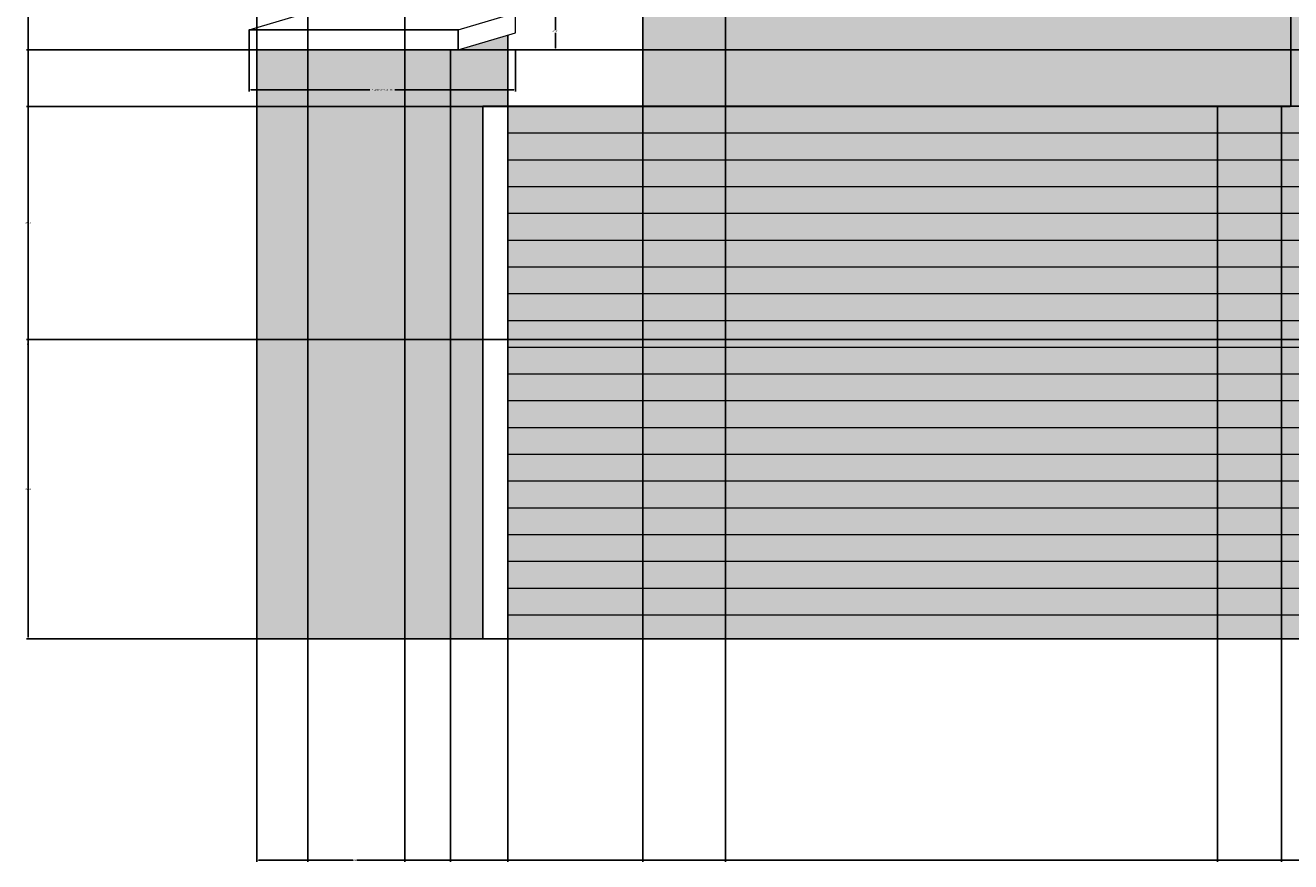
# Model space of a CAD drawing. Units: feet. Extents: x 2926 to 4178, y 965 to 1469.
# Tile 1 of 9: x 2926 to 3068, y 965 to 1059. Entities that reach past the tile are written whole.
import ezdxf

# ---------------------------------------------------------------- set-up
doc = ezdxf.new("R2010")
doc.units = ezdxf.units.FT
for name, color, linetype, lineweight in [('A-ANNO-DIMS', 2, 'Continuous', 18), ('A-ELEV', 7, 'Continuous', 25), ('A-ELEV-DETL', 8, 'Continuous', 18), ('A-ELEV-PATT', 9, 'Continuous', 13)]:
    doc.layers.add(name, color=color, linetype=linetype, lineweight=lineweight)
doc.styles.get("Standard").update_dxf_attribs({"font": 'arial.ttf'})
doc.dimstyles.get("Standard").update_dxf_attribs({"dimtxt": 0.18, "dimasz": 0.18, "dimexe": 0.18, "dimexo": 0.0625, "dimgap": 0.09, "dimtad": 0, "dimtih": 1, "dimtoh": 1, "dimdec": 1, "dimzin": 0, "dimdsep": 46, "dimlunit": 3, "dimtxsty": 'Standard', "dimcen": 0.09, "dimadec": 0, "dimazin": 0, "dimtfac": 1, "dimtdec": 1, "dimtofl": 0, "dimtmove": 0, "dimatfit": 3, "dimfxl": 1, "dimtolj": 1, "dimtzin": 0, "dimarcsym": 0})

# ---------------------------------------------------------------- blocks, each defined once
blk = doc.blocks.new('PILLAR-CAP-A')
for p, q in [((0, 2.25), (6.42, 4.14)), ((0, 2.25), (6.42, 4.14)), ((29.85, 4.14), (6.42, 4.14)), ((29.85, 4.14), (6.42, 4.14)), ((23.43, 2.25), (29.85, 4.14)), ((23.43, 2.25), (29.85, 4.14)), ((29.85, 1.89), (29.85, 4.14)), ((29.85, 1.89), (29.85, 4.14)), ((23.43, 0), (29.85, 1.89)), ((23.43, 0), (29.85, 1.89))]:
    blk.add_line(p, q)
blk = doc.blocks.new('*D6')
at = {"layer": 'A-ANNO-DIMS', "color": 0, "lineweight": -2, "transparency": 16777216}
for p, q in [((2951.55, 1056.26), (2951.55, 1051.66)), ((2981.4, 1056.26), (2981.4, 1051.66)), ((2951.73, 1051.84), (2965.07, 1051.84)), ((2981.22, 1051.84), (2967.88, 1051.84))]:
    blk.add_line(p, q, dxfattribs=at)
at = {"layer": 'A-ANNO-DIMS', "color": 0, "transparency": 16777216}
for points in [[(2951.73, 1051.87), (2951.73, 1051.81), (2951.55, 1051.84)], [(2981.22, 1051.87), (2981.22, 1051.81), (2981.4, 1051.84)]]:
    blk.add_solid(points, dxfattribs=at)
at = {"layer": 'Defpoints', "color": 0, "transparency": 16777216}
for p in [(2951.55, 1056.32), (2981.4, 1056.32), (2981.4, 1051.84)]:
    blk.add_point(p, dxfattribs=at)
at = {"layer": 'A-ANNO-DIMS', "color": 0, "transparency": 16777216, "insert": (2966.48, 1051.84), "char_height": 0.18, "attachment_point": 5}
blk.add_mtext('\\A1;PILLAR CAP A 30 TYP.', dxfattribs=at)
blk = doc.blocks.new('*D7')
at = {"layer": 'A-ANNO-DIMS', "color": 0, "lineweight": -2, "transparency": 16777216}
for p, q in [((2981.46, 1060.46), (2986.06, 1060.46)), ((2985.88, 1060.28), (2985.88, 1058.57)), ((2985.88, 1056.5), (2985.88, 1058.21)), ((2981.46, 1056.32), (2986.06, 1056.32))]:
    blk.add_line(p, q, dxfattribs=at)
at = {"layer": 'A-ANNO-DIMS', "color": 0, "transparency": 16777216}
for points in [[(2985.85, 1060.28), (2985.91, 1060.28), (2985.88, 1060.46)], [(2985.85, 1056.5), (2985.91, 1056.5), (2985.88, 1056.32)]]:
    blk.add_solid(points, dxfattribs=at)
at = {"layer": 'Defpoints', "color": 0, "transparency": 16777216}
for p in [(2981.4, 1060.46), (2985.88, 1060.46), (2981.4, 1056.32)]:
    blk.add_point(p, dxfattribs=at)
at = {"layer": 'A-ANNO-DIMS', "color": 0, "transparency": 16777216, "insert": (2985.88, 1058.39), "char_height": 0.18, "attachment_point": 5}
blk.add_mtext('\\A1;4 TYP.', dxfattribs=at)
blk = doc.blocks.new('*D12')
at = {"layer": 'A-ANNO-DIMS', "color": 0, "lineweight": -2, "transparency": 16777216}
for p, q in [((3335.85, 1023.86), (2926.57, 1023.86)), ((2926.75, 1023.68), (2926.75, 1007.27)), ((2926.75, 990.5), (2926.75, 1006.91)), ((2952.34, 990.32), (2926.57, 990.32))]:
    blk.add_line(p, q, dxfattribs=at)
at = {"layer": 'A-ANNO-DIMS', "color": 0, "transparency": 16777216}
for points in [[(2926.72, 1023.68), (2926.78, 1023.68), (2926.75, 1023.86)], [(2926.72, 990.5), (2926.78, 990.5), (2926.75, 990.32)]]:
    blk.add_solid(points, dxfattribs=at)
at = {"layer": 'Defpoints', "color": 0, "transparency": 16777216}
for p in [(2926.75, 1023.86), (3335.91, 1023.86), (2952.4, 990.32)]:
    blk.add_point(p, dxfattribs=at)
at = {"layer": 'A-ANNO-DIMS', "color": 0, "transparency": 16777216, "insert": (2926.75, 1007.09), "char_height": 0.18, "attachment_point": 5}
blk.add_mtext('\\A1;33.53', dxfattribs=at)
blk = doc.blocks.new('*D13')
at = {"layer": 'A-ANNO-DIMS', "color": 0, "lineweight": -2, "transparency": 16777216}
for p, q in [((3068.25, 1049.98), (2926.57, 1049.98)), ((2926.75, 1049.8), (2926.75, 1037.1)), ((2926.75, 1024.04), (2926.75, 1036.74)), ((3335.85, 1023.86), (2926.57, 1023.86))]:
    blk.add_line(p, q, dxfattribs=at)
at = {"layer": 'A-ANNO-DIMS', "color": 0, "transparency": 16777216}
for points in [[(2926.72, 1049.8), (2926.78, 1049.8), (2926.75, 1049.98)], [(2926.72, 1024.04), (2926.78, 1024.04), (2926.75, 1023.86)]]:
    blk.add_solid(points, dxfattribs=at)
at = {"layer": 'Defpoints', "color": 0, "transparency": 16777216}
for p in [(2926.75, 1049.98), (3068.31, 1049.98), (3335.91, 1023.86)]:
    blk.add_point(p, dxfattribs=at)
at = {"layer": 'A-ANNO-DIMS', "color": 0, "transparency": 16777216, "insert": (2926.75, 1036.92), "char_height": 0.18, "attachment_point": 5}
blk.add_mtext('\\A1;26.13', dxfattribs=at)
blk = doc.blocks.new('*D14')
at = {"layer": 'A-ANNO-DIMS', "color": 0, "lineweight": -2, "transparency": 16777216}
for p, q in [((3068.25, 1092.04), (2926.57, 1092.04)), ((2926.75, 1091.86), (2926.75, 1071.2)), ((2926.75, 1050.16), (2926.75, 1070.83)), ((3068.25, 1049.98), (2926.57, 1049.98))]:
    blk.add_line(p, q, dxfattribs=at)
at = {"layer": 'A-ANNO-DIMS', "color": 0, "transparency": 16777216}
for points in [[(2926.72, 1091.86), (2926.78, 1091.86), (2926.75, 1092.04)], [(2926.72, 1050.16), (2926.78, 1050.16), (2926.75, 1049.98)]]:
    blk.add_solid(points, dxfattribs=at)
at = {"layer": 'Defpoints', "color": 0, "transparency": 16777216}
for p in [(2926.75, 1092.04), (3068.31, 1092.04), (3068.31, 1049.98)]:
    blk.add_point(p, dxfattribs=at)
at = {"layer": 'A-ANNO-DIMS', "color": 0, "transparency": 16777216, "insert": (2926.75, 1071.01), "char_height": 0.18, "attachment_point": 5}
blk.add_mtext('\\A1;42.06', dxfattribs=at)
blk = doc.blocks.new('*D22')
at = {"layer": 'A-ANNO-DIMS', "color": 0, "lineweight": -2, "transparency": 16777216}
for p, q in [((2952.4, 1056.38), (2952.4, 1468.62)), ((2952.58, 1468.44), (3009.97, 1468.44)), ((3068.13, 1468.44), (3010.74, 1468.44)), ((3068.31, 1050.05), (3068.31, 1468.62))]:
    blk.add_line(p, q, dxfattribs=at)
at = {"layer": 'A-ANNO-DIMS', "color": 0, "transparency": 16777216}
for points in [[(2952.58, 1468.47), (2952.58, 1468.41), (2952.4, 1468.44)], [(3068.13, 1468.47), (3068.13, 1468.41), (3068.31, 1468.44)]]:
    blk.add_solid(points, dxfattribs=at)
at = {"layer": 'Defpoints', "color": 0, "transparency": 16777216}
for p in [(3068.31, 1468.44), (2952.4, 1056.32), (3068.31, 1049.98)]:
    blk.add_point(p, dxfattribs=at)
at = {"layer": 'A-ANNO-DIMS', "color": 0, "transparency": 16777216, "insert": (3010.36, 1468.44), "char_height": 0.18, "attachment_point": 5}
blk.add_mtext('\\A1;115.9', dxfattribs=at)
blk = doc.blocks.new('*D23')
at = {"layer": 'A-ANNO-DIMS', "color": 0, "lineweight": -2, "transparency": 16777216}
for p, q in [((3068.31, 1050.05), (3068.31, 1468.62)), ((3068.49, 1468.44), (3099.11, 1468.44)), ((3130.51, 1468.44), (3099.9, 1468.44)), ((3130.69, 1050.05), (3130.69, 1468.62))]:
    blk.add_line(p, q, dxfattribs=at)
at = {"layer": 'A-ANNO-DIMS', "color": 0, "transparency": 16777216}
for points in [[(3068.49, 1468.47), (3068.49, 1468.41), (3068.31, 1468.44)], [(3130.51, 1468.47), (3130.51, 1468.41), (3130.69, 1468.44)]]:
    blk.add_solid(points, dxfattribs=at)
at = {"layer": 'Defpoints', "color": 0, "transparency": 16777216}
for p in [(3130.69, 1468.44), (3068.31, 1049.98), (3130.69, 1049.98)]:
    blk.add_point(p, dxfattribs=at)
at = {"layer": 'A-ANNO-DIMS', "color": 0, "transparency": 16777216, "insert": (3099.5, 1468.44), "char_height": 0.18, "attachment_point": 5}
blk.add_mtext('\\A1;62.38', dxfattribs=at)
blk = doc.blocks.new('*D50')
at = {"layer": 'A-ANNO-DIMS', "color": 0, "lineweight": -2, "transparency": 16777216}
for p, q in [((2952.4, 1171.83), (2952.4, 965.34)), ((2958.11, 1170.16), (2958.11, 965.34)), ((2952.58, 965.52), (2954.87, 965.52)), ((2957.93, 965.52), (2955.65, 965.52))]:
    blk.add_line(p, q, dxfattribs=at)
at = {"layer": 'A-ANNO-DIMS', "color": 0, "transparency": 16777216}
for points in [[(2952.58, 965.55), (2952.58, 965.49), (2952.4, 965.52)], [(2957.93, 965.55), (2957.93, 965.49), (2958.11, 965.52)]]:
    blk.add_solid(points, dxfattribs=at)
at = {"layer": 'Defpoints', "color": 0, "transparency": 16777216}
for p in [(2952.4, 1171.9), (2958.11, 1170.22), (2958.11, 965.52)]:
    blk.add_point(p, dxfattribs=at)
at = {"layer": 'A-ANNO-DIMS', "color": 0, "transparency": 16777216, "insert": (2955.26, 965.52), "char_height": 0.18, "attachment_point": 5}
blk.add_mtext('\\A1;5.712', dxfattribs=at)
blk = doc.blocks.new('*D51')
at = {"layer": 'A-ANNO-DIMS', "color": 0, "lineweight": -2, "transparency": 16777216}
for p, q in [((2958.11, 1170.16), (2958.11, 965.34)), ((2968.99, 1170.16), (2968.99, 965.34)), ((2958.29, 965.52), (2963.11, 965.52)), ((2968.81, 965.52), (2963.99, 965.52))]:
    blk.add_line(p, q, dxfattribs=at)
at = {"layer": 'A-ANNO-DIMS', "color": 0, "transparency": 16777216}
for points in [[(2958.29, 965.55), (2958.29, 965.49), (2958.11, 965.52)], [(2968.81, 965.55), (2968.81, 965.49), (2968.99, 965.52)]]:
    blk.add_solid(points, dxfattribs=at)
at = {"layer": 'Defpoints', "color": 0, "transparency": 16777216}
for p in [(2958.11, 1170.22), (2968.99, 1170.22), (2968.99, 965.52)]:
    blk.add_point(p, dxfattribs=at)
at = {"layer": 'A-ANNO-DIMS', "color": 0, "transparency": 16777216, "insert": (2963.55, 965.52), "char_height": 0.18, "attachment_point": 5}
blk.add_mtext('\\A1;10.871', dxfattribs=at)
blk = doc.blocks.new('*D52')
at = {"layer": 'A-ANNO-DIMS', "color": 0, "lineweight": -2, "transparency": 16777216}
for p, q in [((2968.99, 1170.16), (2968.99, 965.34)), ((2995.67, 1170.16), (2995.67, 965.34)), ((2969.17, 965.52), (2981.86, 965.52)), ((2995.49, 965.52), (2982.79, 965.52))]:
    blk.add_line(p, q, dxfattribs=at)
at = {"layer": 'A-ANNO-DIMS', "color": 0, "transparency": 16777216}
for points in [[(2969.17, 965.55), (2969.17, 965.49), (2968.99, 965.52)], [(2995.49, 965.55), (2995.49, 965.49), (2995.67, 965.52)]]:
    blk.add_solid(points, dxfattribs=at)
at = {"layer": 'Defpoints', "color": 0, "transparency": 16777216}
for p in [(2968.99, 1170.22), (2995.67, 1170.22), (2995.67, 965.52)]:
    blk.add_point(p, dxfattribs=at)
at = {"layer": 'A-ANNO-DIMS', "color": 0, "transparency": 16777216, "insert": (2982.33, 965.52), "char_height": 0.18, "attachment_point": 5}
blk.add_mtext('\\A1;26.685', dxfattribs=at)
blk = doc.blocks.new('*D53')
at = {"layer": 'A-ANNO-DIMS', "color": 0, "lineweight": -2, "transparency": 16777216}
for p, q in [((3004.93, 1228.4), (3004.93, 965.34)), ((2995.67, 1170.16), (2995.67, 965.34)), ((2995.85, 965.52), (2999.91, 965.52)), ((3004.75, 965.52), (3000.69, 965.52))]:
    blk.add_line(p, q, dxfattribs=at)
at = {"layer": 'A-ANNO-DIMS', "color": 0, "transparency": 16777216}
for points in [[(2995.85, 965.55), (2995.85, 965.49), (2995.67, 965.52)], [(3004.75, 965.55), (3004.75, 965.49), (3004.93, 965.52)]]:
    blk.add_solid(points, dxfattribs=at)
at = {"layer": 'Defpoints', "color": 0, "transparency": 16777216}
for p in [(3004.93, 1228.46), (2995.67, 1170.22), (3004.93, 965.52)]:
    blk.add_point(p, dxfattribs=at)
at = {"layer": 'A-ANNO-DIMS', "color": 0, "transparency": 16777216, "insert": (3000.3, 965.52), "char_height": 0.18, "attachment_point": 5}
blk.add_mtext('\\A1;9.257', dxfattribs=at)
blk = doc.blocks.new('*D54')
at = {"layer": 'A-ANNO-DIMS', "color": 0, "lineweight": -2, "transparency": 16777216}
for p, q in [((3004.93, 1228.4), (3004.93, 965.34)), ((3084.03, 1170.16), (3084.03, 965.34)), ((3005.11, 965.52), (3044.17, 965.52)), ((3083.85, 965.52), (3044.79, 965.52))]:
    blk.add_line(p, q, dxfattribs=at)
at = {"layer": 'A-ANNO-DIMS', "color": 0, "transparency": 16777216}
for points in [[(3005.11, 965.55), (3005.11, 965.49), (3004.93, 965.52)], [(3083.85, 965.55), (3083.85, 965.49), (3084.03, 965.52)]]:
    blk.add_solid(points, dxfattribs=at)
at = {"layer": 'Defpoints', "color": 0, "transparency": 16777216}
for p in [(3004.93, 1228.46), (3084.03, 1170.22), (3084.03, 965.52)]:
    blk.add_point(p, dxfattribs=at)
at = {"layer": 'A-ANNO-DIMS', "color": 0, "transparency": 16777216, "insert": (3044.48, 965.52), "char_height": 0.18, "attachment_point": 5}
blk.add_mtext('\\A1;79.1', dxfattribs=at)
blk = doc.blocks.new('*D66')
at = {"layer": 'A-ANNO-DIMS', "color": 0, "lineweight": -2, "transparency": 16777216}
for p, q in [((2952.4, 990.26), (2952.4, 965.34)), ((2974.12, 990.26), (2974.12, 965.34)), ((2952.58, 965.52), (2962.87, 965.52)), ((2973.94, 965.52), (2963.66, 965.52))]:
    blk.add_line(p, q, dxfattribs=at)
at = {"layer": 'A-ANNO-DIMS', "color": 0, "transparency": 16777216}
for points in [[(2952.58, 965.55), (2952.58, 965.49), (2952.4, 965.52)], [(2973.94, 965.55), (2973.94, 965.49), (2974.12, 965.52)]]:
    blk.add_solid(points, dxfattribs=at)
at = {"layer": 'Defpoints', "color": 0, "transparency": 16777216}
for p in [(2952.4, 990.32), (2974.12, 990.32), (2974.12, 965.52)]:
    blk.add_point(p, dxfattribs=at)
at = {"layer": 'A-ANNO-DIMS', "color": 0, "transparency": 16777216, "insert": (2963.26, 965.52), "char_height": 0.18, "attachment_point": 5}
blk.add_mtext('\\A1;21.72', dxfattribs=at)
blk = doc.blocks.new('*D67')
at = {"layer": 'A-ANNO-DIMS', "color": 0, "lineweight": -2, "transparency": 16777216}
for p, q in [((2974.12, 990.26), (2974.12, 965.34)), ((2980.53, 990.26), (2980.53, 965.34)), ((2974.3, 965.52), (2976.93, 965.52)), ((2980.35, 965.52), (2977.72, 965.52))]:
    blk.add_line(p, q, dxfattribs=at)
at = {"layer": 'A-ANNO-DIMS', "color": 0, "transparency": 16777216}
for points in [[(2974.3, 965.55), (2974.3, 965.49), (2974.12, 965.52)], [(2980.35, 965.55), (2980.35, 965.49), (2980.53, 965.52)]]:
    blk.add_solid(points, dxfattribs=at)
at = {"layer": 'Defpoints', "color": 0, "transparency": 16777216}
for p in [(2974.12, 990.32), (2980.53, 990.32), (2980.53, 965.52)]:
    blk.add_point(p, dxfattribs=at)
at = {"layer": 'A-ANNO-DIMS', "color": 0, "transparency": 16777216, "insert": (2977.33, 965.52), "char_height": 0.18, "attachment_point": 5}
blk.add_mtext('\\A1;6.406', dxfattribs=at)
blk = doc.blocks.new('*D68')
at = {"layer": 'A-ANNO-DIMS', "color": 0, "lineweight": -2, "transparency": 16777216}
for p, q in [((2980.53, 990.26), (2980.53, 965.34)), ((3060.1, 990.26), (3060.1, 965.34)), ((2980.71, 965.52), (3019.92, 965.52)), ((3059.92, 965.52), (3020.71, 965.52))]:
    blk.add_line(p, q, dxfattribs=at)
at = {"layer": 'A-ANNO-DIMS', "color": 0, "transparency": 16777216}
for points in [[(2980.71, 965.55), (2980.71, 965.49), (2980.53, 965.52)], [(3059.92, 965.55), (3059.92, 965.49), (3060.1, 965.52)]]:
    blk.add_solid(points, dxfattribs=at)
at = {"layer": 'Defpoints', "color": 0, "transparency": 16777216}
for p in [(2980.53, 990.32), (3060.1, 990.32), (3060.1, 965.52)]:
    blk.add_point(p, dxfattribs=at)
at = {"layer": 'A-ANNO-DIMS', "color": 0, "transparency": 16777216, "insert": (3020.32, 965.52), "char_height": 0.18, "attachment_point": 5}
blk.add_mtext('\\A1;79.57', dxfattribs=at)
blk = doc.blocks.new('*D69')
at = {"layer": 'A-ANNO-DIMS', "color": 0, "lineweight": -2, "transparency": 16777216}
for p, q in [((3060.1, 990.26), (3060.1, 965.34)), ((3067.27, 990.26), (3067.27, 965.34)), ((3060.28, 965.52), (3063.29, 965.52)), ((3067.09, 965.52), (3064.08, 965.52))]:
    blk.add_line(p, q, dxfattribs=at)
at = {"layer": 'A-ANNO-DIMS', "color": 0, "transparency": 16777216}
for points in [[(3060.28, 965.55), (3060.28, 965.49), (3060.1, 965.52)], [(3067.09, 965.55), (3067.09, 965.49), (3067.27, 965.52)]]:
    blk.add_solid(points, dxfattribs=at)
at = {"layer": 'Defpoints', "color": 0, "transparency": 16777216}
for p in [(3060.1, 990.32), (3067.27, 990.32), (3067.27, 965.52)]:
    blk.add_point(p, dxfattribs=at)
at = {"layer": 'A-ANNO-DIMS', "color": 0, "transparency": 16777216, "insert": (3063.69, 965.52), "char_height": 0.18, "attachment_point": 5}
blk.add_mtext('\\A1;7.169', dxfattribs=at)
blk = doc.blocks.new('*D70')
at = {"layer": 'A-ANNO-DIMS', "color": 0, "lineweight": -2, "transparency": 16777216}
for p, q in [((3067.27, 990.26), (3067.27, 965.34)), ((3146.65, 990.26), (3146.65, 965.34)), ((3067.45, 965.52), (3106.57, 965.52)), ((3146.47, 965.52), (3107.35, 965.52))]:
    blk.add_line(p, q, dxfattribs=at)
at = {"layer": 'A-ANNO-DIMS', "color": 0, "transparency": 16777216}
for points in [[(3067.45, 965.55), (3067.45, 965.49), (3067.27, 965.52)], [(3146.47, 965.55), (3146.47, 965.49), (3146.65, 965.52)]]:
    blk.add_solid(points, dxfattribs=at)
at = {"layer": 'Defpoints', "color": 0, "transparency": 16777216}
for p in [(3067.27, 990.32), (3146.65, 990.32), (3146.65, 965.52)]:
    blk.add_point(p, dxfattribs=at)
at = {"layer": 'A-ANNO-DIMS', "color": 0, "transparency": 16777216, "insert": (3106.96, 965.52), "char_height": 0.18, "attachment_point": 5}
blk.add_mtext('\\A1;79.38', dxfattribs=at)
blk = doc.blocks.new('*D73')
at = {"layer": 'A-ANNO-DIMS', "color": 0, "lineweight": -2, "transparency": 16777216}
for p, q in [((3174.15, 1056.32), (2926.57, 1056.32)), ((2926.75, 1056.14), (2926.75, 1023.5)), ((2926.75, 990.5), (2926.75, 1023.14)), ((3174.15, 990.32), (2926.57, 990.32))]:
    blk.add_line(p, q, dxfattribs=at)
at = {"layer": 'A-ANNO-DIMS', "color": 0, "transparency": 16777216}
for points in [[(2926.72, 1056.14), (2926.78, 1056.14), (2926.75, 1056.32)], [(2926.72, 990.5), (2926.78, 990.5), (2926.75, 990.32)]]:
    blk.add_solid(points, dxfattribs=at)
at = {"layer": 'Defpoints', "color": 0, "transparency": 16777216}
for p in [(2926.75, 1056.32), (3174.22, 1056.32), (3174.22, 990.32)]:
    blk.add_point(p, dxfattribs=at)
at = {"layer": 'A-ANNO-DIMS', "color": 0, "transparency": 16777216, "insert": (2926.75, 1023.32), "char_height": 0.18, "attachment_point": 5}
blk.add_mtext('\\A1;66', dxfattribs=at)

msp = doc.modelspace()

# ---------------------------------------------------------------- hatches: boundary and pattern name
at = {"layer": 'A-ELEV-PATT'}
h = msp.add_hatch(color=256, dxfattribs=at)
h.dxf.hatch_style = 1
h.paths.add_polyline_path([(3006.649, 1296.2176), (2952.4018, 1296.2176), (2952.4018, 1252.1389), (3006.649, 1252.1389)])
h.paths.add_polyline_path([(3084.0314, 1226.8042), (3008.2802, 1226.8042), (3008.2802, 1171.8963), (3084.0314, 1171.8963)])
h.paths.add_polyline_path([(3004.9276, 1228.4641), (2995.6704, 1228.4641), (2995.6704, 1171.8963), (3004.9276, 1171.8963)])
h.paths.add_polyline_path([(3174.217, 1236.3246), (3084.0314, 1236.3246), (3084.0314, 1171.8963), (3124.7575, 1171.8963), (3124.7575, 1207.1083), (3154.7729, 1207.1083), (3154.7729, 1171.8963), (3174.217, 1171.8963)])
h.paths.add_polyline_path([(3273.5987, 1236.3246), (3174.217, 1236.3246), (3174.217, 1171.8963), (3174.217, 1126.1389), (3174.217, 1116.3246), (3273.5987, 1116.3246)], flags=16)
h.paths.add_polyline_path([(3198.6415, 1219.2195), (3244.819, 1219.2195), (3244.819, 1133.2879), (3198.6415, 1133.2879)], flags=0)
h.paths.add_polyline_path([(3432.4018, 1427.8302), (3174.217, 1427.8302), (3174.217, 1356.4366), (3174.5501, 1355.2778), (3221.3497, 1355.2778), (3221.3497, 1364.3965), (3232.8063, 1364.3965), (3232.8063, 1355.2778), (3236.4098, 1355.2778), (3236.4098, 1364.3965), (3247.8663, 1364.3965), (3247.8663, 1355.2778), (3250.7081, 1355.2778), (3250.7081, 1364.3965), (3262.1646, 1364.3965), (3262.1646, 1355.2778), (3379.9311, 1355.2778), (3379.9311, 990.3246), (3432.4018, 990.3246)])
h.paths.add_polyline_path([(3068.3128, 1092.0439), (3130.6886, 1092.0439), (3130.6886, 1049.9841), (3146.6469, 1049.9841), (3146.6469, 1057.7915), (3145.2184, 1058.2122), (3145.2184, 1060.462), (3168.644, 1060.462), (3174.217, 1058.8204), (3174.217, 1110.3246), (3004.9276, 1110.3246), (3004.9276, 1049.9841), (3068.3128, 1049.9841)])
h.paths.add_polyline_path([(3174.217, 1056.3197), (3152.4954, 1056.3197), (3152.4954, 990.3246), (3174.217, 990.3246)])
h.paths.add_polyline_path([(2974.1234, 1056.3197), (2952.4018, 1056.3197), (2952.4018, 990.3246), (2974.1234, 990.3246)])
h.paths.add_polyline_path([(3004.9276, 1110.3246), (2995.6704, 1110.3246), (2995.6704, 1049.9841), (3004.9276, 1049.9841)])
h = msp.add_hatch(color=256, dxfattribs=at)
h.dxf.hatch_style = 1
h.paths.add_polyline_path([(3174.217, 1297.8963), (3172.3488, 1297.8963), (3006.649, 1297.8963), (3006.649, 1296.2176), (3087.9974, 1296.2176), (3087.9974, 1252.1389), (3089.8656, 1252.1389), (3089.8656, 1296.2176), (3172.3488, 1296.2176), (3172.3488, 1252.1389), (3174.217, 1252.1389)])
h.paths.add_polyline_path([(3102.4583, 1170.2176), (3172.3488, 1170.2176), (3172.3488, 1126.1389), (3174.217, 1126.1389), (3174.217, 1171.8963), (3172.3488, 1171.8963), (2952.4018, 1171.8963), (2952.4018, 1170.2176), (2952.4018, 1126.1389), (2954.27, 1126.1389), (2954.27, 1170.2176), (3100.5901, 1170.2176), (3100.5901, 1126.1389), (3102.4583, 1126.1389)])
h.paths.add_polyline_path([(3130.6886, 1092.0439), (3068.3128, 1092.0439), (3068.3128, 1049.9841), (3130.6886, 1049.9841)])
h.paths.add_polyline_path([(3099.0016, 1090.4638), (3099.0016, 1051.5643), (3069.893, 1051.5643), (3069.893, 1090.4638)], flags=16)
h.paths.add_polyline_path([(3099.9998, 1090.4638), (3129.1085, 1090.4638), (3129.1085, 1051.5643), (3099.9998, 1051.5643)], flags=16)
h.paths.add_polyline_path([(3067.2712, 1049.9841), (3060.102, 1049.9841), (3060.102, 990.3246), (3067.2712, 990.3246)])
h.paths.add_polyline_path([(3339.7517, 1326.907), (3364.1168, 1326.907), (3364.1168, 1330.7444), (3335.9143, 1330.7444), (3335.9143, 1023.8561), (3364.1168, 1023.8561), (3364.1168, 1027.6935), (3339.7517, 1027.6935)])
h.paths.add_polyline_path([(3154.7729, 1207.1083), (3124.7575, 1207.1083), (3124.7575, 1171.8963), (3126.8684, 1171.8963), (3126.8684, 1204.9974), (3152.6619, 1204.9974), (3152.6619, 1171.8963), (3154.7729, 1171.8963)])
h = msp.add_hatch(color=256, dxfattribs=at)
h.dxf.hatch_style = 1
h.paths.add_polyline_path([(2980.5295, 1057.9557), (2974.9754, 1056.3197), (2974.1234, 1056.3197), (2974.1234, 990.3246), (2977.7283, 990.3246), (2977.7283, 1049.9841), (2980.5295, 1049.9841)])
h.paths.add_polyline_path([(3152.4954, 1056.3197), (3151.6434, 1056.3197), (3146.6469, 1057.7915), (3146.6469, 1049.9841), (3149.6449, 1049.9841), (3149.6449, 990.3246), (3152.4954, 990.3246)])
h.paths.add_polyline_path([(3008.2802, 1226.8042), (3004.9276, 1228.4641), (3004.9276, 1171.8963), (3008.2802, 1171.8963)])
h = msp.add_hatch(color=256, dxfattribs=at)
h.dxf.hatch_style = 1
h.paths.add_polyline_path([(3146.6469, 1049.9841), (2980.5295, 1049.9841), (2980.5295, 990.3246), (3146.6469, 990.3246)])
h = msp.add_hatch(dxfattribs=at)
h.set_pattern_fill('_USER', color=256, scale=3, pattern_type=0)
h.set_pattern_definition([(0, (0, 0), (0, 3), [])])
h.paths.add_polyline_path([(3146.6469, 1049.9841), (2980.5295, 1049.9841), (2980.5295, 990.3246), (3146.6469, 990.3246)])

# ---------------------------------------------------------------- linework, layer by layer
at = {"layer": 'A-ELEV'}
for p, q in [((2980.5295, 1057.9557), (2980.5295, 990.3246)), ((2980.5295, 1057.9557), (2980.5295, 990.3246)), ((2952.4018, 990.3246), (2952.4018, 1056.3197)), ((2952.4018, 990.3246), (2952.4018, 1056.3197)), ((2952.4018, 990.3246), (3432.4018, 990.3246)), ((2952.4018, 990.3246), (3432.4018, 990.3246))]:
    msp.add_line(p, q, dxfattribs=at)
for points in [[(2995.6704, 1110.3246), (3004.9276, 1110.3246), (3004.9276, 1049.9841), (2995.6704, 1049.9841)], [(2995.6704, 1110.3246), (3004.9276, 1110.3246), (3004.9276, 1049.9841), (2995.6704, 1049.9841)], [(2951.5498, 1056.3197), (2974.9754, 1056.3197), (2974.9754, 1058.5694), (2951.5498, 1058.5694)], [(2951.5498, 1056.3197), (2974.9754, 1056.3197), (2974.9754, 1058.5694), (2951.5498, 1058.5694)], [(2974.1234, 990.3246), (2952.4018, 990.3246), (2952.4018, 1056.3197), (2974.1234, 1056.3197)], [(2974.1234, 990.3246), (2952.4018, 990.3246), (2952.4018, 1056.3197), (2974.1234, 1056.3197)], [(2977.7283, 1049.9841), (3149.6449, 1049.9841), (3149.6449, 990.3246), (2977.7283, 990.3246)], [(2977.7283, 1049.9841), (3149.6449, 1049.9841), (3149.6449, 990.3246), (2977.7283, 990.3246)], [(3060.102, 1049.9841), (3067.2712, 1049.9841), (3067.2712, 990.3246), (3060.102, 990.3246)]]:
    msp.add_lwpolyline(points, close=True, dxfattribs=at)

# ---------------------------------------------------------------- block references
at = {"layer": 'A-ELEV-DETL'}
msp.add_blockref('PILLAR-CAP-A', (2951.55, 1056.32), dxfattribs=at)

# ---------------------------------------------------------------- dimensions: what is measured, and where the dimension line sits
at = {"layer": 'A-ANNO-DIMS'}
for base, p1, p2, override, picture, middle in [((3068.3128, 1468.4445), (2952.4018, 1056.3197), (3068.3128, 1049.9841), {"dimdec": 1, "dimlfac": 1, "dimrnd": 0, "dimzin": 0, "dimdsep": 46, "dimlunit": 2}, '*D22', (3010.3573, 1468.4445)), ((3130.6886, 1468.4445), (3068.3128, 1049.9841), (3130.6886, 1049.9841), {"dimdec": 2, "dimlfac": 1, "dimrnd": 0, "dimzin": 0, "dimdsep": 46, "dimlunit": 2}, '*D23', (3099.5007, 1468.4445)), ((3004.9276, 965.5246), (2995.6704, 1170.2176), (3004.9276, 1228.4641), {"dimdec": 3, "dimlfac": 1, "dimrnd": 0, "dimzin": 0, "dimdsep": 46, "dimlunit": 2}, '*D53', (3000.299, 965.5246)), ((3084.0314, 965.5246), (3004.9276, 1228.4641), (3084.0314, 1170.2176), {"dimdec": 1, "dimlfac": 1, "dimrnd": 0, "dimzin": 0, "dimdsep": 46, "dimlunit": 2}, '*D54', (3044.4795, 965.5246)), ((2958.1139, 965.5246), (2952.4018, 1171.8963), (2958.1139, 1170.2176), {"dimdec": 3, "dimlfac": 1, "dimrnd": 0, "dimzin": 0, "dimdsep": 46, "dimlunit": 2}, '*D50', (2955.2579, 965.5246)), ((2968.9852, 965.5246), (2958.1139, 1170.2176), (2968.9852, 1170.2176), {"dimdec": 3, "dimlfac": 1, "dimrnd": 0, "dimzin": 0, "dimdsep": 46, "dimlunit": 2}, '*D51', (2963.5496, 965.5246)), ((2995.6704, 965.5246), (2968.9852, 1170.2176), (2995.6704, 1170.2176), {"dimdec": 3, "dimlfac": 1, "dimrnd": 0, "dimzin": 0, "dimdsep": 46, "dimlunit": 2}, '*D52', (2982.3278, 965.5246)), ((2974.1234, 965.5246), (2952.4018, 990.3246), (2974.1234, 990.3246), {"dimdec": 2, "dimlfac": 1, "dimrnd": 0, "dimzin": 0, "dimdsep": 46, "dimlunit": 2}, '*D66', (2963.2626, 965.5246)), ((2980.5295, 965.5246), (2974.1234, 990.3246), (2980.5295, 990.3246), {"dimdec": 3, "dimlfac": 1, "dimrnd": 0, "dimzin": 0, "dimdsep": 46, "dimlunit": 2}, '*D67', (2977.3265, 965.5246)), ((3060.102, 965.5246), (2980.5295, 990.3246), (3060.102, 990.3246), {"dimdec": 2, "dimlfac": 1, "dimrnd": 0, "dimzin": 0, "dimdsep": 46, "dimlunit": 2}, '*D68', (3020.3158, 965.5246)), ((3067.2712, 965.5246), (3060.102, 990.3246), (3067.2712, 990.3246), {"dimdec": 3, "dimlfac": 1, "dimrnd": 0, "dimzin": 0, "dimdsep": 46, "dimlunit": 2}, '*D69', (3063.6866, 965.5246)), ((3146.6469, 965.5246), (3067.2712, 990.3246), (3146.6469, 990.3246), {"dimdec": 2, "dimlfac": 1, "dimrnd": 0, "dimzin": 0, "dimdsep": 46, "dimlunit": 2}, '*D70', (3106.959, 965.5246))]:
    dim = msp.add_linear_dim(base=base, p1=p1, p2=p2, dimstyle='Standard', override=override, dxfattribs=at)
    dim.commit()
    dim.dimension.update_dxf_attribs({"geometry": picture, "text_midpoint": middle})
for base, p1, p2, override, picture, middle in [((2926.7498, 1092.0439), (3068.3128, 1049.9841), (3068.3128, 1092.0439), {"dimdec": 2, "dimlfac": 1, "dimrnd": 0, "dimzin": 0, "dimdsep": 46, "dimlunit": 2}, '*D14', (2926.7498, 1071.014)), ((2926.7498, 1056.3197), (3174.217, 990.3246), (3174.217, 1056.3197), {"dimdec": 0, "dimlfac": 1, "dimrnd": 0, "dimzin": 0, "dimdsep": 46, "dimlunit": 2}, '*D73', (2926.7498, 1023.3221)), ((2926.7498, 1049.9841), (3335.9143, 1023.8561), (3068.3128, 1049.9841), {"dimdec": 2, "dimlfac": 1, "dimrnd": 0, "dimzin": 0, "dimdsep": 46, "dimlunit": 2}, '*D13', (2926.7498, 1036.9201)), ((2926.7498, 1023.8561), (2952.4018, 990.3246), (3335.9143, 1023.8561), {"dimdec": 2, "dimlfac": 1, "dimrnd": 0, "dimzin": 0, "dimdsep": 46, "dimlunit": 2}, '*D12', (2926.7498, 1007.0903))]:
    dim = msp.add_linear_dim(base=base, p1=p1, p2=p2, angle=90, dimstyle='Standard', override=override, dxfattribs=at)
    dim.commit()
    dim.dimension.update_dxf_attribs({"geometry": picture, "text_midpoint": middle})
dim = msp.add_linear_dim(base=(2985.878, 1060.462), p1=(2981.4004, 1056.3197), p2=(2981.4004, 1060.462), angle=90, text='<> TYP.', dimstyle='Standard', override={"dimdec": 0, "dimlfac": 1, "dimrnd": 0, "dimzin": 0, "dimdsep": 46, "dimlunit": 2}, dxfattribs=at)
dim.commit()
dim.dimension.update_dxf_attribs({"geometry": '*D7', "text_midpoint": (2985.878, 1058.3908)})
dim = msp.add_linear_dim(base=(2981.4004, 1051.8421), p1=(2951.5498, 1056.3197), p2=(2981.4004, 1056.3197), text='PILLAR CAP A <> TYP.', dimstyle='Standard', override={"dimdec": 0, "dimlfac": 1, "dimrnd": 0, "dimzin": 0, "dimdsep": 46, "dimlunit": 2}, dxfattribs=at)
dim.commit()
dim.dimension.update_dxf_attribs({"geometry": '*D6', "text_midpoint": (2966.4751, 1051.8421)})

doc.saveas('drawing.dxf')
